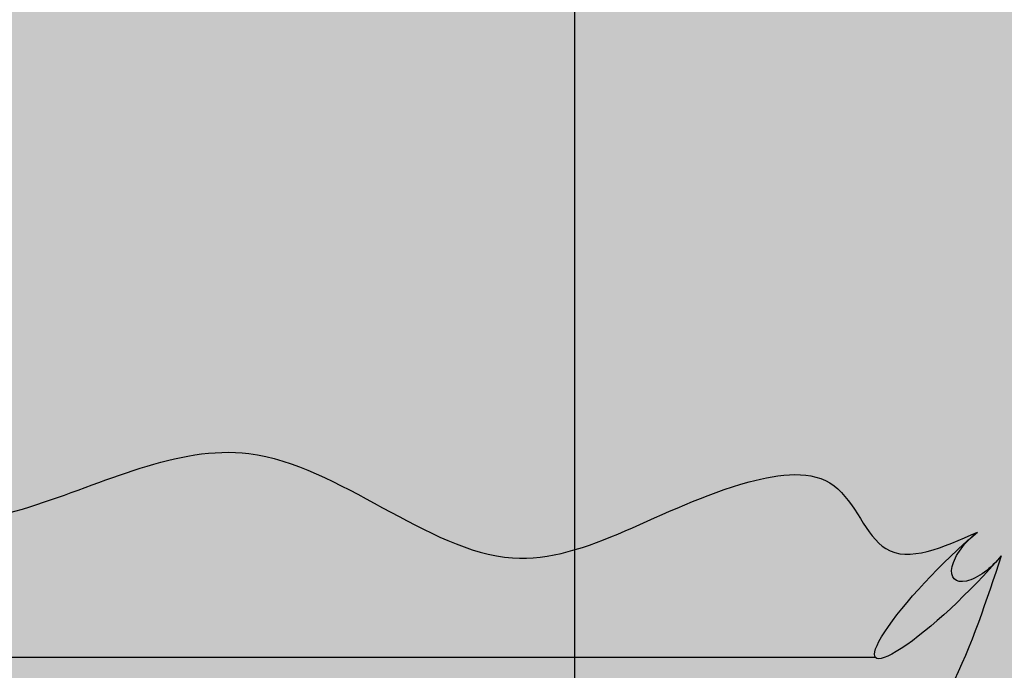
# Model space of a CAD drawing. Units: inches. Extents: x 1704 to 6393, y -157 to 1172.
# Tile 36 of 122: x 2526 to 2564, y 190 to 215. Entities that reach past the tile are written whole.
import ezdxf

# ---------------------------------------------------------------- set-up
doc = ezdxf.new("R2010")
doc.units = ezdxf.units.IN
doc.header["$MEASUREMENT"] = 0
for name, color, linetype, lineweight in [('A-ANNO-DIMS', 7, 'Continuous', 13), ('A-FURN', 8, 'Continuous', 18), ('estofado', 7, 'Continuous', 25)]:
    doc.layers.add(name, color=color, linetype=linetype, lineweight=lineweight)
doc.layers.add('A-FLOR-PATT', color=7, linetype='Continuous', lineweight=13, true_color=0xf2f2f2)
doc.styles.get("Standard").update_dxf_attribs({"font": 'arial.ttf'})
doc.dimstyles.get("Standard").update_dxf_attribs({"dimtxt": 6, "dimasz": 2, "dimexe": 0.18, "dimexo": 0.0625, "dimgap": 0.09, "dimtad": 0, "dimtih": 1, "dimtoh": 1, "dimdec": 1, "dimzin": 0, "dimdsep": 46, "dimlunit": 3, "dimtxsty": 'Standard', "dimblk": 'ARCHTICK', "dimcen": 0.09, "dimadec": 0, "dimazin": 0, "dimtfac": 1, "dimtdec": 1, "dimtofl": 0, "dimtmove": 0, "dimatfit": 3, "dimfxl": 1, "dimtolj": 1, "dimtzin": 0, "dimarcsym": 0})

# ---------------------------------------------------------------- blocks, each defined once
blk = doc.blocks.new('Cama Box Regencia LOLA')
at = {"layer": 'estofado', "ltscale": 0.2}
h = blk.add_hatch(color=256, dxfattribs=at)
h.dxf.hatch_style = 1
h.set_gradient(color1=(206, 178, 131), color2=(233, 221, 200), one_color=1, tint=0.8500000238418579, name='CURVED')
edge = h.paths.add_edge_path()
edge.add_spline(control_points=[(0.9233883396182136, -2.254908822900802), (0.9143712174658276, -2.237158585978875), (0.8971704820246486, -2.20329887728792), (0.9295105801843419, -2.140290914518345), (0.848651568119294, -2.10957861148239), (0.9047062348403186, -2.046222426005954), (0.8299480774321636, -1.990932361540615), (0.9387479200587449, -1.92692496801726), (0.8590435458045249, -1.86767849203585), (0.8322262745575699, -1.826028043643361), (0.8247981799574972, -1.810442049687992)], knot_values=[0, 0, 0, 0, 0.0575832900035364, 0.1098437972159638, 0.1698138218664432, 0.2255174829302509, 0.2824861515521905, 0.3632291183773252, 0.4509842065695901, 0.5012091817853866, 0.5012091817853866, 0.5012091817853866, 0.5012091817853866], degree=3, periodic=0)
edge.add_spline(control_points=[(0.8247981799572698, -1.810442049688447), (0.8512430237993839, -1.769990096378137), (0.8869160776755506, -1.705010622333873), (0.9070359522544322, -1.586338752195842), (0.8536462472426364, -1.488247672851343), (0.8944567470317679, -1.387739666353695), (0.8643796102055603, -1.342420998864781), (0.8547271521993025, -1.327877176513538)], knot_values=[0, 0, 0, 0, 0.1438744691785906, 0.2224893870322766, 0.3492927143212738, 0.4561786976395368, 0.5066917301592304, 0.5066917301592304, 0.5066917301592304, 0.5066917301592304], degree=3, periodic=0)
edge.add_spline(control_points=[(0.8547271521993025, -1.327877176513538), (0.7873766543807506, -1.256744909425322), (0.6449024721503065, -1.106270719748692), (0.3977250465933366, -1.412092721352792), (0.0338148848931041, -1.279726484458706), (-0.3488365122128698, -1.179158668568902), (-0.6188339616464873, -1.25080943574278), (-0.7460155200169539, -1.321708019985464)], knot_values=[0.0991852523588446, 0.0991852523588446, 0.0991852523588446, 0.0991852523588446, 0.3453008654366167, 0.6198216521345741, 0.9826525916749167, 1.386093159660275, 1.810554634340498, 1.810554634340498, 1.810554634340498, 1.810554634340498], degree=3, periodic=0)
edge.add_spline(control_points=[(-0.7460155199962628, -1.32170802000337), (-0.8056354908857201, -1.352141651537124), (-0.8226532004149476, -1.367823298399059), (-0.8348745804664758, -1.38184410903591)], knot_values=[0.0062456970656236, 0.0062456970656236, 0.0062456970656236, 0.0062456970656236, 0.0554759259147193, 0.0554759259147193, 0.0554759259147193, 0.0554759259147193], degree=3, periodic=0)
edge.add_spline(control_points=[(-0.8348745804664758, -1.38184410903591), (-0.8364250716851984, -1.383622888820184), (-0.8378983647115774, -1.385374937005849), (-0.8393716577378427, -1.387126985191514)], knot_values=[0, 0, 0, 0, 0.0062456970656236, 0.0062456970656236, 0.0062456970656236, 0.0062456970656236], degree=3, periodic=0)
edge.add_arc((-0.6180450437709624, -1.576392779500167), 0.2912164331649039, 139.4648411061637, 203.3711573294546)
edge.add_arc((-0.7011750866292914, -1.609837078845487), 0.2016528082906132, 204.0179006417974, 212.6189639884946)
edge.add_spline(control_points=[(-0.8710220093900034, -1.718537943240505), (-0.8696870122217887, -1.721658691442996), (-0.8597709916446092, -1.746046247230935), (-0.8464685798230674, -1.804421032451443), (-0.888988689927828, -1.889951451602371), (-0.8378676506146121, -1.973422824210047), (-0.8371590179440318, -2.05992368952792), (-0.8871569320951948, -2.144598622072578), (-0.908935644436724, -2.210906123939594), (-0.9233883398977695, -2.254908823284267)], knot_values=[0, 0, 0, 0, 0.0101500649009363, 0.0785829584511912, 0.1732273504791735, 0.2688802694005398, 0.3498050162211252, 0.4202002266429896, 0.5590752189863636, 0.5590752189863636, 0.5590752189863636, 0.5590752189863636], degree=3, periodic=0)
edge.add_ellipse((-0.9040800600764669, -2.258882422916315), major_axis=(0.0267880171833212, 0.0267880171833213), ratio=0.4535320972039226, start_angle=94.15910660291303, end_angle=123.37101895145429, ccw=False)
edge.add_ellipse((-0.8772920428931456, -2.232094405732993), major_axis=(0.0772920428927364, 0.0772920428927364), ratio=0.168252450050839, start_angle=-1.0527401173021644e-10, end_angle=156.3071135567154, ccw=False)
edge.add_line((-0.8000000000002955, -2.154802362840428), (0.7999592378284888, -2.154802362840428))
edge.add_arc((0.9462065466516378, -2.098298447668867), 0.1567831871334379, 200.9447658774159, 201.1244713640487, ccw=False)
edge.add_arc((1.115979327553759, -2.004946707326951), 0.3497136727815615, 205.2898146244752, 205.3730108333857)
edge.add_ellipse((0.8772920428930319, -2.232094405732993), major_axis=(-0.0772920428927364, 0.0772920428927364), ratio=0.168252450050839, start_angle=203.6928864432847, end_angle=359.99999999994674, ccw=False)
edge.add_ellipse((0.9040800600763532, -2.258882422916315), major_axis=(-0.0267880171833213, 0.0267880171833213), ratio=0.4535320972039226, start_angle=236.6289810485458, end_angle=265.84089339708703, ccw=False)
h = blk.add_hatch(color=256, dxfattribs=at)
h.dxf.hatch_style = 1
h.set_gradient(color1=(206, 178, 131), color2=(233, 221, 200), one_color=1, tint=0.8500000238418579, name='CURVED')
edge = h.paths.add_edge_path()
edge.add_ellipse((-0.8772920428931456, -2.232094405732993), major_axis=(0.0772920428927364, 0.0772920428927364), ratio=0.168252450050839, start_angle=-156.3071135577263, end_angle=-1.05349e-10)
edge.add_ellipse((-0.8772920428931456, -2.232094405732993), major_axis=(0.0772920428927364, 0.0772920428927364), ratio=0.168252450050839, start_angle=-1.05349e-10, end_angle=156.3071135567153)
edge.add_ellipse((-0.9040800600764669, -2.258882422916315), major_axis=(0.0267880171833212, 0.0267880171833213), ratio=0.4535320972039226, start_angle=-94.15910660848522, end_angle=94.15910660291303, ccw=False)
h = blk.add_hatch(color=256, dxfattribs=at)
h.dxf.hatch_style = 1
h.set_gradient(color1=(206, 178, 131), color2=(233, 221, 200), one_color=1, tint=0.8500000238418579, name='CURVED')
edge = h.paths.add_edge_path()
edge.add_spline(control_points=[(-0.9001064604443627, -2.27819070273756), (-0.866259371332262, -2.263084355976445), (-0.8028331991894219, -2.234776522858453), (-0.7685206103102474, -2.343981002846874), (-0.6122536186376238, -2.322828464485212), (-0.4353754265674752, -2.183795504726106), (-0.2043351766035357, -2.412166101990749), (0.035742157155596, -2.28434544697319), (0.2724023732024534, -2.265741378418681), (0.4990197572961961, -2.339647395113615), (0.6925408411253784, -2.202138696866825), (0.8240737498149427, -2.250332331133733), (0.900106460444249, -2.27819070273756)], knot_values=[0, 0, 0, 0, 0.0915194039844232, 0.1714985135733706, 0.2551966802733756, 0.4993431682155844, 0.7776132872898075, 0.9991109890269537, 1.23769004728933, 1.492615491211055, 1.658192352121012, 1.885025012049534, 1.885025012049534, 1.885025012049534, 1.885025012049534], degree=3, periodic=0)
edge.add_ellipse((0.9040800600763532, -2.258882422916315), major_axis=(-0.0267880171833213, 0.0267880171833213), ratio=0.4535320972039226, start_angle=454.1591066084853, end_angle=483.3710189511271, ccw=False)
edge.add_ellipse((0.8772920428930319, -2.232094405732993), major_axis=(-0.0772920428927364, 0.0772920428927364), ratio=0.168252450050839, start_angle=359.99999999994674, end_angle=516.3071135577263, ccw=False)
edge.add_arc((0.9462065466977946, -2.098298447788181), 0.1567831871334379, 201.1244713173118, 201.142614633458, ccw=False)
edge.add_line((0.7999592378286025, -2.154802362840428), (-0.8000000000004092, -2.154802362840428))
edge.add_ellipse((-0.8772920428931456, -2.232094405732993), major_axis=(0.0772920428927364, 0.0772920428927364), ratio=0.168252450050839, start_angle=-156.3071135577261, end_angle=-1.0527401173021644e-10, ccw=False)
edge.add_ellipse((-0.9040800600764669, -2.258882422916315), major_axis=(0.0267880171833212, 0.0267880171833213), ratio=0.4535320972039226, start_angle=-123.3710189511271, end_angle=-94.15910660848522, ccw=False)
blk.add_line((-0.7999999999999546, -2.154802362840428), (0.8000000000000682, -2.154802362840428), dxfattribs=at)
at = {"layer": 'estofado', "ltscale": 0.2, "extrusion": (0, 0, -1)}
for centre, major_axis, ratio, start_param, end_param in [((-0.8772920428931456, -2.232094405732993), (0.0772920428927364, 0.0772920428927364), 0.168252450050839, 4.250341947992563, 8.31602866635556), ((-0.9040800600764669, -2.258882422916315), (0.0267880171833212, 0.0267880171833213), 0.4535320972039226, 4.422106649467695, 8.144263964888069)]:
    blk.add_ellipse(centre, major_axis=major_axis, ratio=ratio, start_param=start_param, end_param=end_param, dxfattribs=at)
at = {"layer": 'estofado', "ltscale": 0.2}
for points, knots in [([(-0.9233883398977695, -2.254908823284267), (-0.908935644436724, -2.210906123939594), (-0.8871569320951948, -2.144598622072578), (-0.8371590179440318, -2.05992368952792), (-0.8378676506146121, -1.973422824210047), (-0.888988689927828, -1.889951451602371), (-0.8464685798230674, -1.804421032451443), (-0.8597709916446092, -1.746046247230935), (-0.8696870122217887, -1.721658691442996), (-0.8710220093900034, -1.718537943240505)], [0, 0, 0, 0, 0.1388749923433741, 0.2092702027652384, 0.2901949495858238, 0.3858478685071901, 0.4804922605351724, 0.5489251540854273, 0.5590752189863636, 0.5590752189863636, 0.5590752189863636, 0.5590752189863636]), ([(0.900106460444249, -2.27819070273756), (0.8240737498147286, -2.250332331133789), (0.6925408411252015, -2.202138696866918), (0.4990197572963532, -2.33964739511349), (0.2724023732023884, -2.265741378418779), (0.0357421571555867, -2.284345446973105), (-0.204335176603578, -2.412166101990773), (-0.4353754265674596, -2.183795504726199), (-0.6122536186375224, -2.322828464485116), (-0.7685206103102122, -2.343981002846907), (-0.8028331991894692, -2.234776522858419), (-0.8662593713322198, -2.263084355976456), (-0.9001064604443627, -2.27819070273756)], [0, 0, 0, 0, 0.2268326599285221, 0.3924095208384793, 0.6473349647602045, 0.8859140230225809, 1.107411724759727, 1.38568184383395, 1.629828331776159, 1.713526498476164, 1.793505608065111, 1.885025012049534, 1.885025012049534, 1.885025012049534, 1.885025012049534])]:
    blk.add_open_spline(points, degree=3, knots=knots, dxfattribs=at)
blk = doc.blocks.new('_ArchTick')
at = {"color": 0, "linetype": 'ByBlock', "const_width": 0.15}
blk.add_lwpolyline([(-0.5, -0.5), (0.5, 0.5)], dxfattribs=at)
blk = doc.blocks.new('*D93')
at = {"layer": 'A-ANNO-DIMS', "color": 0, "lineweight": -2, "transparency": 16777216}
for p, q in [((2605.286074000001, 895.2129740000005), (1829.697551000002, 895.2129740000003)), ((1829.877551000002, 895.2129740000003), (1829.877551000002, 495.8664119263302)), ((1829.877551000002, 90.2129739999999), (1829.877551000002, 489.5595360736699)), ((2605.286074000001, 90.21297400000003), (1829.697551000002, 90.2129739999999))]:
    blk.add_line(p, q, dxfattribs=at)
at = {"layer": 'Defpoints', "color": 0, "lineweight": -3, "transparency": 16777216}
for p in [(2605.348574000001, 895.2129740000005), (1829.877551000002, 90.2129739999999), (2605.348574000001, 90.21297400000003)]:
    blk.add_point(p, dxfattribs=at)
at = {"layer": 'A-ANNO-DIMS', "color": 0, "lineweight": -2, "transparency": 16777216, "xscale": 2, "yscale": 2, "zscale": 2}
for p, rotation in [((1829.877551000002, 895.2129740000003), 90), ((1829.877551000002, 90.2129739999999), 270)]:
    blk.add_blockref('_ArchTick', p, dxfattribs=dict(at, rotation=rotation))
at = {"layer": 'A-ANNO-DIMS', "color": 0, "transparency": 16777216, "insert": (1829.877551000001, 492.7129739999994), "char_height": 6, "attachment_point": 5}
blk.add_mtext('\\A1;805', dxfattribs=at)
blk = doc.blocks.new('*D105')
at = {"layer": 'A-ANNO-DIMS', "color": 0, "lineweight": -2, "transparency": 16777216}
for p, q in [((2451.737975, 615.150474), (2451.737975, -64.9670259999999)), ((2547.348574, 615.150474), (2547.348574, -64.9670259999999)), ((2451.737975, -64.787026), (2489.908936164393, -64.787026)), ((2547.348574, -64.787026), (2509.177612835607, -64.787026))]:
    blk.add_line(p, q, dxfattribs=at)
at = {"layer": 'Defpoints', "color": 0, "lineweight": -3, "transparency": 16777216}
for p in [(2451.737975, 615.212974), (2547.348574, 615.212974), (2547.348574, -64.787026)]:
    blk.add_point(p, dxfattribs=at)
at = {"layer": 'A-ANNO-DIMS', "color": 0, "lineweight": -2, "transparency": 16777216, "xscale": 2, "yscale": 2, "zscale": 2, "rotation": 180}
blk.add_blockref('_ArchTick', (2451.737975, -64.787026), dxfattribs=at)
at = {"layer": 'A-ANNO-DIMS', "color": 0, "lineweight": -2, "transparency": 16777216, "xscale": 2, "yscale": 2, "zscale": 2}
blk.add_blockref('_ArchTick', (2547.348574, -64.787026), dxfattribs=at)
at = {"layer": 'A-ANNO-DIMS', "color": 0, "transparency": 16777216, "insert": (2499.5432745, -64.787026), "char_height": 6, "attachment_point": 5}
blk.add_mtext('\\A1;95.61', dxfattribs=at)

msp = doc.modelspace()

# ---------------------------------------------------------------- hatches: boundary and pattern name
at = {"layer": 'A-FLOR-PATT', "transparency": 33554528}
h = msp.add_hatch(color=256, dxfattribs=at)
h.dxf.hatch_style = 1
h.paths.add_polyline_path([(2325.348574056059, 863.2129735309796), (2325.348574056059, 887.2129735309796), (2263.348574056059, 887.2129735309796), (2167.348574056059, 887.2129735309794), (2081.348574056061, 887.2129735309792), (2081.348574056061, 719.2129735309785), (2277.348574056059, 719.2129735309787), (2277.348574056059, 711.2129735309788), (2277.348574056059, 372.212973530979), (2349.348574056059, 372.212973530979), (2381.348574056059, 372.2129735309789), (2381.348574056059, 364.2129735309789), (2353.348574056059, 364.2129735309789), (2353.348574056059, 270.2129735309788), (2381.348574056059, 270.2129735309788), (2381.348574056059, 266.2129735309788), (2357.348574056059, 266.2129735309788), (2357.348574056059, 98.21297353097884), (2381.348574056059, 98.21297353097897), (2385.181056550604, 98.21297353097884), (2386.482186711948, 98.21297353097884), (2424.21496140017, 98.21297353097884), (2425.516091561514, 98.21297353097884), (2429.348574056059, 98.21297353097897), (2597.348574056059, 98.21297353097884), (2597.348574056059, 146.2129735309788), (2597.348574056059, 218.2129735309788), (2597.348574056059, 266.2129735309788), (2423.348574056059, 266.2129735309788), (2423.348574056059, 270.2129735309788), (2473.348574056059, 270.2129735309788), (2473.348574056059, 294.2129735309789), (2477.348574056059, 294.2129735309789), (2477.348574056059, 270.2129735309788), (2547.348574056059, 270.2129735309788), (2547.348574056059, 364.2129735309788), (2477.348574056059, 364.2129735309788), (2477.348574056059, 318.2129735309788), (2473.348574056059, 318.2129735309787), (2473.348574056059, 364.2129735309789), (2423.348574056059, 364.2129735309788), (2423.348574056059, 372.2129735309788), (2469.348574056059, 372.2129735309788), (2469.348574056059, 459.2129735309789), (2469.348574056059, 538.2129735309788), (2350.348574056059, 538.2129735309788), (2350.348574056059, 565.7129735309788), (2358.348574056059, 565.7129735309788), (2358.348574056059, 545.2129735309788), (2420.348574056059, 545.2129735309788), (2420.348574056059, 610.2129735309788), (2358.348574056059, 610.2129735309788), (2358.348574056059, 589.7129735309788), (2350.348574056059, 589.7129735309788), (2350.348574056059, 615.2129735309788), (2425.348574056059, 615.2129735309788), (2425.348574056059, 607.2129735309788), (2425.348574056059, 546.2129735309788), (2469.348574056059, 546.2129735309788), (2514.34857405606, 546.212973530979), (2514.34857405606, 607.2129735309788), (2449.348574056059, 607.2129735309788), (2449.348574056059, 615.2129735309788), (2451.737974987759, 615.2129735309788), (2451.737974987759, 659.2129735309788), (2427.737974987759, 659.2129735309788), (2427.737974987759, 665.2129735309788), (2367.737974987758, 665.2129735309788), (2367.737974987758, 667.2129735309788), (2367.737974987758, 711.2129735309788), (2325.348574056059, 711.2129735309788), (2325.348574056059, 719.2129735309785), (2325.348574056059, 755.2129735309787), (2325.348574056059, 763.2129735309788)])
h.paths.add_polyline_path([(2233.85817000392, 822.532660166629, -0.1872470486944155), (2233.85817000392, 809.1396667958562), (2231.697030374885, 808.8044951349628, 0.0848927708004382), (2233.130501812631, 814.4858417746204), (2230.423974436808, 814.4858417746204, -0.1042581087707907), (2228.553363812687, 808.3129425443484), (2217.750790159711, 807.1555239386723, -0.2222222222222219), (2217.750790159711, 824.5168030238124), (2228.553363812687, 823.3593844181363, -0.1042581087707933), (2230.423974436808, 817.1864851878643), (2233.130501812631, 817.1864851878643, 0.08489277080044), (2231.697030374885, 822.8678318275219)], flags=16)
h.paths.add_polyline_path([(2213.621360876743, 833.1974425663823), (2213.621360876743, 798.4748843961024), (2156.047684459484, 798.4748843961034), (2156.047684459485, 833.1974425663813)], flags=16)
h.paths.add_polyline_path([(2203.931929661768, 848.0987249710489), (2205.089348267444, 837.2961513180724, -0.2222222222222264), (2187.728069182304, 837.2961513180724), (2188.88548778798, 848.0987249710485, -0.104258108770792), (2195.058387018252, 849.9693355951691), (2195.058387018252, 852.6758629709927, 0.084892770800438), (2189.377040378595, 851.2423915332469), (2189.712212039488, 853.4035311622828, -0.1872470486944166), (2203.105205410261, 853.4035311622828), (2203.440377071154, 851.2423915332469, 0.084892770800438), (2197.759030431496, 852.6758629709927), (2197.759030431496, 849.9693355951691, -0.1042581087707896)], flags=16)
h.paths.add_polyline_path([(2181.940976153924, 837.2961513180726, -0.2222222222222323), (2164.579697068783, 837.2961513180724), (2165.73711567446, 848.0987249710487, -0.1042581087707905), (2171.910014904732, 849.9693355951691), (2171.910014904732, 852.6758629709927, 0.0848927708004445), (2166.228668265074, 851.2423915332469), (2166.563839925967, 853.403531162283, -0.1872470486944096), (2179.95683329674, 853.4035311622828), (2180.292004957633, 851.2423915332465, 0.0848927708004458), (2174.610658317976, 852.6758629709927), (2174.610658317976, 849.9693355951691, -0.104258108770801), (2180.783557548248, 848.0987249710482)], flags=16)
h.paths.add_polyline_path([(2205.089348267444, 794.376175644412), (2203.931929661768, 783.5736019914364, -0.1042581087707934), (2197.759030431496, 781.7029913673155), (2197.759030431496, 778.9964639914921, 0.084892770800439), (2203.440377071154, 780.4299354292382), (2203.105205410261, 778.2687958002022, -0.1872470486944172), (2189.712212039488, 778.2687958002018), (2189.377040378595, 780.4299354292377, 0.0848927708004369), (2195.058387018252, 778.9964639914919), (2195.058387018252, 781.7029913673153, -0.1042581087707904), (2188.88548778798, 783.5736019914358), (2187.728069182304, 794.3761756444126, -0.2222222222222231)], flags=16)
h.paths.add_polyline_path([(2181.940976153924, 794.376175644412), (2180.783557548248, 783.5736019914364, -0.1042581087708008), (2174.610658317976, 781.7029913673153), (2174.610658317976, 778.9964639914921, 0.0848927708004458), (2180.292004957633, 780.4299354292382), (2179.95683329674, 778.268795800202, -0.1872470486944096), (2166.563839925967, 778.2687958002018), (2166.228668265074, 780.4299354292378, 0.0848927708004446), (2171.910014904732, 778.9964639914919), (2171.910014904732, 781.7029913673153, -0.1042581087707904), (2165.73711567446, 783.5736019914358), (2164.579697068783, 794.3761756444123, -0.2222222222222294)], flags=16)
h.paths.add_polyline_path([(2151.918255176517, 807.1555239386723), (2141.115681523541, 808.3129425443484, -0.1042581087707911), (2139.24507089942, 814.4858417746204), (2136.538543523597, 814.4858417746204, 0.08489277080044), (2137.972014961343, 808.8044951349626), (2135.810875332307, 809.1396667958562, -0.1872470486944109), (2135.810875332307, 822.5326601666285), (2137.972014961343, 822.8678318275221, 0.0848927708004416), (2136.538543523597, 817.1864851878643), (2139.24507089942, 817.1864851878643, -0.104258108770793), (2141.115681523541, 823.3593844181363), (2151.918255176517, 824.5168030238124, -0.2222222222222205)], flags=16)
h.paths.add_polyline_path([(2357.868011454448, 363.4102250290031), (2358.813881560335, 363.4102250290031, 0.7537604849588476)], flags=16)
h.paths.add_polyline_path([(2372.241054283868, 363.1167008961685), (2372.248110816919, 363.1167008961685), (2372.248110816919, 363.3425764997267), (2371.30224071103, 363.3425764997267), (2371.30224071103, 363.1392706554335, -1.360391292333951)], flags=16)
h.paths.add_polyline_path([(2371.309297244092, 272.7157694655011), (2371.30224071103, 272.7157694655011), (2371.30224071103, 272.4898938619428), (2372.248110816919, 272.4898938619428), (2372.248110816919, 272.6931997062759, -1.360391292393621)], flags=16)
h.paths.add_polyline_path([(2357.875067987504, 272.7157694655011), (2357.868011454452, 272.7157694655011), (2357.868011454452, 272.4898938619428), (2358.813881560341, 272.4898938619428), (2358.813881560341, 272.6931997062361, -1.360391292333948)], flags=16)
h.paths.add_polyline_path([(2353.768696905258, 363.0736921025416), (2376.347425366111, 363.0736921025416), (2376.347425366111, 272.7587782591281), (2353.768696905258, 272.7587782591281)], flags=16)
h.paths.add_polyline_path([(2354.772195947961, 362.0701930598379), (2375.343926323407, 362.0701930598379), (2375.343926323407, 273.7622773018316), (2354.772195947961, 273.7622773018318)], flags=0)
h.paths.add_polyline_path([(2357.868011454452, 363.3425764997267), (2358.813881560341, 363.3425764997266), (2358.813881560341, 363.1167008961684), (2357.868011454452, 363.1167008961684)], flags=16)
h.paths.add_polyline_path([(2359.287941640134, 359.1843485433627), (2359.287941640134, 360.0631949744305), (2370.828180631237, 360.0631949744362), (2370.828180631237, 359.1843485433769), (2374.332057422314, 359.1843485433812), (2374.332057422312, 358.4635369582513), (2372.835178716611, 358.4635369582524), (2372.835178716611, 357.5410357047662), (2374.332057422314, 357.5410357047678), (2374.332057422312, 356.8202241196381), (2372.835178716611, 356.820224119639), (2372.835178716611, 355.897722866153), (2374.332057422314, 355.8977228661546), (2374.332057422312, 355.1769112810248), (2372.835178716611, 355.1769112810259), (2372.835178716611, 354.2544100275397), (2374.332057422334, 354.2544100275415), (2374.332057422331, 353.5335984424117), (2372.835178716631, 353.5335984424126), (2372.835178716631, 352.6110971889265), (2374.332057422334, 352.6110971889282), (2374.332057422331, 351.8902856037984), (2372.835178716631, 351.8902856037993), (2372.835178716631, 350.9677843503132), (2374.332057422334, 350.967784350315), (2374.332057422331, 350.2469727651852), (2372.835178716631, 350.2469727651861), (2372.835178716631, 349.3244715117), (2374.332057422334, 349.3244715117017), (2374.332057422331, 348.603659926572), (2372.835178716631, 348.6036599265729), (2372.835178716631, 347.6811586730868), (2374.332057422334, 347.6811586730886), (2374.332057422331, 346.9603470879587), (2372.835178716631, 346.9603470879598), (2372.835178716631, 346.0378458344735), (2374.332057422334, 346.0378458344753), (2374.332057422331, 345.3170342493456), (2372.835178716631, 345.3170342493465), (2372.835178716631, 344.3945329958605), (2374.332057422334, 344.3945329958621), (2374.332057422331, 343.6737214107324), (2372.835178716631, 343.6737214107334), (2372.835178716631, 342.751220157247), (2374.332057422334, 342.7512201572489), (2374.332057422331, 342.0304085721191), (2372.835178716631, 342.03040857212), (2372.835178716631, 341.1079073186338), (2374.332057422334, 341.1079073186356), (2374.332057422331, 340.3870957335057), (2372.835178716631, 340.3870957335066), (2372.835178716631, 339.4645944800207), (2374.332057422334, 339.4645944800223), (2374.332057422331, 338.7437828948924), (2372.835178716648, 338.7437828948933), (2372.835178716648, 337.8212816414076), (2374.332057422334, 337.8212816414093), (2374.332057422331, 337.1004700562794), (2372.835178716648, 337.1004700562803), (2372.835178716648, 336.1779688027942), (2374.332057422334, 336.1779688027961), (2374.332057422331, 335.4571572176662), (2372.835178716648, 335.4571572176673), (2372.835178716648, 334.5346559641809), (2374.332057422334, 334.5346559641828), (2374.332057422331, 333.8138443790529), (2372.835178716648, 333.8138443790539), (2372.835178716648, 332.8913431255679), (2374.332057422334, 332.8913431255696), (2374.332057422331, 332.1705315404397), (2372.835178716648, 332.1705315404406), (2372.835178716648, 331.2480302869545), (2374.332057422334, 331.2480302869563), (2374.332057422331, 330.5272187018265), (2372.835178716648, 330.5272187018273), (2372.835178716648, 329.6047174483413), (2374.332057422334, 329.6047174483431), (2374.332057422331, 328.8839058632133), (2372.835178716648, 328.8839058632143), (2372.835178716648, 327.9614046097282), (2374.332057422334, 327.9614046097298), (2374.332057422331, 327.2405930246), (2372.835178716648, 327.2405930246009), (2372.835178716648, 326.3180917711149), (2374.332057422334, 326.3180917711167), (2374.332057422331, 325.5972801859869), (2372.835178716648, 325.5972801859877), (2372.835178716648, 324.6747789325016), (2374.332057422334, 324.6747789325034), (2374.332057422331, 323.9539673473736), (2372.835178716648, 323.9539673473746), (2372.835178716648, 323.0314660938884), (2374.332057422334, 323.0314660938901), (2374.332057422331, 322.3106545087603), (2372.835178716648, 322.3106545087613), (2372.835178716648, 321.3881532552753), (2374.332057422334, 321.388153255277), (2374.332057422331, 320.6673416701471), (2372.835178716648, 320.6673416701481), (2372.835178716648, 319.7448404166621), (2374.332057422334, 319.7448404166638), (2374.332057422331, 319.0240288315339), (2372.835178716648, 319.0240288315348), (2372.835178716648, 318.1015275780487), (2374.332057422334, 318.1015275780504), (2374.332057422331, 317.3807159929205), (2372.835178716648, 317.3807159929214), (2372.835178716648, 316.4582147394357), (2374.332057422334, 316.4582147394373), (2374.332057422331, 315.7374031543073), (2372.835178716648, 315.7374031543084), (2372.835178716648, 314.8149019008223), (2374.332057422334, 314.8149019008241), (2374.332057422331, 314.0940903156943), (2372.835178716648, 314.0940903156952), (2372.835178716648, 313.171589062209), (2374.332057422334, 313.1715890622108), (2374.332057422331, 312.450777477081), (2372.835178716648, 312.4507774770819), (2372.835178716648, 311.5282762235959), (2374.332057422334, 311.5282762235977), (2374.332057422331, 310.8074646384678), (2372.835178716648, 310.8074646384687), (2372.835178716648, 309.8849633849827), (2374.332057422334, 309.8849633849844), (2374.332057422331, 309.1641517998546), (2372.835178716648, 309.1641517998555), (2372.835178716648, 308.2416505463693), (2374.332057422334, 308.2416505463712), (2374.332057422331, 307.5208389612412), (2372.835178716648, 307.5208389612421), (2372.835178716648, 306.5983377077562), (2374.332057422334, 306.598337707758), (2374.332057422331, 305.8775261226281), (2372.835178716648, 305.8775261226289), (2372.835178716648, 304.955024869143), (2374.332057422334, 304.9550248691447), (2374.332057422331, 304.2342132840149), (2372.835178716648, 304.2342132840158), (2372.835178716648, 303.3117120305298), (2374.332057422334, 303.3117120305316), (2374.332057422331, 302.5909004454018), (2372.835178716648, 302.5909004454027), (2372.835178716648, 301.6683991919165), (2374.332057422334, 301.6683991919183), (2374.332057422331, 300.9475876067885), (2372.835178716648, 300.9475876067894), (2372.835178716648, 300.0250863533033), (2374.332057422334, 300.025086353305), (2374.332057422331, 299.3042747681752), (2372.835178716648, 299.3042747681761), (2372.835178716648, 298.3817735146902), (2374.332057422334, 298.3817735146919), (2374.332057422331, 297.6609619295621), (2372.835178716648, 297.6609619295629), (2372.835178716648, 296.7384606760769), (2374.332057422334, 296.7384606760786), (2374.332057422331, 296.0176490909488), (2372.835178716648, 296.0176490909498), (2372.835178716648, 295.0951478374636), (2374.332057422334, 295.0951478374653), (2374.332057422331, 294.3743362523355), (2372.835178716648, 294.3743362523364), (2372.835178716648, 293.4518349988504), (2374.332057422334, 293.4518349988522), (2374.332057422331, 292.7310234137224), (2372.835178716648, 292.7310234137233), (2372.835178716648, 291.8085221602371), (2374.332057422334, 291.8085221602389), (2374.332057422331, 291.0877105751091), (2372.835178716648, 291.08771057511), (2372.835178716648, 290.165209321624), (2374.332057422334, 290.1652093216256), (2374.332057422331, 289.4443977364957), (2372.835178716648, 289.4443977364966), (2372.835178716648, 288.5218964830108), (2374.332057422334, 288.5218964830125), (2374.332057422331, 287.8010848978827), (2372.835178716648, 287.8010848978836), (2372.835178716648, 286.8785836443975), (2374.332057422334, 286.8785836443993), (2374.332057422331, 286.1577720592695), (2372.835178716648, 286.1577720592703), (2372.835178716648, 285.2352708057842), (2374.332057422334, 285.2352708057861), (2374.332057422331, 284.5144592206562), (2372.835178716648, 284.514459220657), (2372.835178716648, 283.5919579671712), (2374.332057422334, 283.5919579671728), (2374.332057422331, 282.871146382043), (2372.835178716648, 282.8711463820439), (2372.835178716648, 281.9486451285579), (2374.332057422334, 281.9486451285596), (2374.332057422331, 281.2278335434298), (2372.835178716648, 281.2278335434307), (2372.835178716648, 280.3053322899446), (2374.332057422334, 280.3053322899464), (2374.332057422331, 279.5845207048164), (2372.835178716648, 279.5845207048174), (2372.835178716648, 278.6620194513314), (2374.332057422334, 278.6620194513331), (2374.332057422331, 277.9412078662033), (2372.835178716648, 277.9412078662043), (2372.835178716648, 277.0187066127184), (2374.332057422334, 277.0187066127201), (2374.332057422331, 276.29789502759), (2370.828180631244, 276.2978950275922), (2370.828180631244, 275.7692753872335), (2359.287941640128, 275.7692753872392), (2359.287941640128, 276.2978950275993), (2355.784064849037, 276.2978950276015), (2355.784064849037, 277.0187066126971), (2357.280943554723, 277.0187066126989), (2357.280943554723, 277.9412078662137), (2355.784064849037, 277.9412078662145), (2355.784064849037, 278.6620194513103), (2357.280943554723, 278.6620194513122), (2357.280943554723, 279.5845207048271), (2355.784064849037, 279.584520704828), (2355.784064849037, 280.3053322899236), (2357.280943554723, 280.3053322899253), (2357.280943554723, 281.2278335434403), (2355.784064849037, 281.2278335434412), (2355.784064849037, 281.9486451285369), (2357.280943554723, 281.9486451285387), (2357.280943554723, 282.8711463820535), (2355.784064849037, 282.8711463820543), (2355.784064849037, 283.5919579671501), (2357.280943554723, 283.591957967152), (2357.280943554723, 284.5144592206668), (2355.784064849037, 284.5144592206676), (2355.784064849037, 285.2352708057632), (2357.280943554723, 285.2352708057651), (2357.280943554723, 286.1577720592801), (2355.784064849037, 286.1577720592809), (2355.784064849037, 286.8785836443766), (2357.280943554723, 286.8785836443784), (2357.280943554723, 287.8010848978931), (2355.784064849037, 287.8010848978941), (2355.784064849037, 288.5218964829895), (2357.280943554723, 288.5218964829913), (2357.280943554723, 289.4443977365064), (2355.784064849037, 289.4443977365072), (2355.784064849037, 290.1652093216029), (2357.280943554723, 290.1652093216047), (2357.280943554723, 291.0877105751197), (2355.784064849037, 291.0877105751206), (2355.784064849037, 291.8085221602161), (2357.280943554723, 291.8085221602179), (2357.280943554723, 292.7310234137328), (2355.784064849037, 292.7310234137337), (2355.784064849037, 293.4518349988293), (2357.280943554723, 293.451834998831), (2357.280943554723, 294.3743362523461), (2355.784064849037, 294.3743362523469), (2355.784064849037, 295.0951478374426), (2357.280943554723, 295.0951478374445), (2357.280943554723, 296.0176490909594), (2355.784064849037, 296.0176490909601), (2355.784064849037, 296.7384606760557), (2357.280943554723, 296.7384606760575), (2357.280943554723, 297.6609619295724), (2355.784064849037, 297.6609619295734), (2355.784064849037, 298.3817735146691), (2357.280943554723, 298.3817735146709), (2357.280943554723, 299.3042747681858), (2355.784064849037, 299.3042747681866), (2355.784064849037, 300.0250863532823), (2357.280943554723, 300.0250863532841), (2357.280943554723, 300.9475876067989), (2355.784064849037, 300.9475876067997), (2355.784064849037, 301.6683991918954), (2357.280943554723, 301.6683991918973), (2357.280943554723, 302.5909004454123), (2355.784064849037, 302.5909004454133), (2355.784064849037, 303.3117120305088), (2357.280943554723, 303.3117120305105), (2357.280943554723, 304.2342132840254), (2355.784064849037, 304.2342132840262), (2355.784064849037, 304.9550248691219), (2357.280943554723, 304.9550248691238), (2357.280943554723, 305.8775261226386), (2355.784064849037, 305.8775261226394), (2355.784064849037, 306.5983377077352), (2357.280943554723, 306.5983377077369), (2357.280943554723, 307.5208389612518), (2355.784064849037, 307.5208389612528), (2355.784064849037, 308.2416505463484), (2357.280943554723, 308.2416505463501), (2357.280943554723, 309.1641517998652), (2355.784064849037, 309.1641517998661), (2355.784064849037, 309.8849633849617), (2357.280943554723, 309.8849633849634), (2357.280943554723, 310.8074646384782), (2355.784064849037, 310.8074646384791), (2355.784064849037, 311.5282762235748), (2357.280943554723, 311.5282762235767), (2357.280943554723, 312.4507774770916), (2355.784064849037, 312.4507774770925), (2355.784064849037, 313.171589062188), (2357.280943554723, 313.1715890621898), (2357.280943554723, 314.0940903157049), (2355.784064849037, 314.0940903157058), (2355.784064849037, 314.8149019008013), (2357.280943554723, 314.8149019008032), (2357.280943554723, 315.7374031543179), (2355.784064849037, 315.7374031543187), (2355.784064849037, 316.4582147394146), (2357.280943554723, 316.4582147394165), (2357.280943554723, 317.3807159929311), (2355.784064849037, 317.3807159929321), (2355.784064849037, 318.1015275780277), (2357.280943554723, 318.1015275780295), (2357.280943554723, 319.0240288315445), (2355.784064849037, 319.0240288315454), (2355.784064849037, 319.744840416641), (2357.280943554723, 319.7448404166428), (2357.280943554723, 320.6673416701576), (2355.784064849037, 320.6673416701585), (2355.784064849037, 321.3881532552541), (2357.280943554723, 321.388153255256), (2357.280943554723, 322.3106545087708), (2355.784064849037, 322.3106545087718), (2355.784064849037, 323.0314660938674), (2357.280943554723, 323.0314660938692), (2357.280943554723, 323.9539673473843), (2355.784064849037, 323.9539673473851), (2355.784064849037, 324.6747789324806), (2357.280943554723, 324.6747789324824), (2357.280943554723, 325.5972801859974), (2355.784064849037, 325.5972801859983), (2355.784064849037, 326.3180917710939), (2357.280943554723, 326.3180917710958), (2357.280943554723, 327.2405930246105), (2355.784064849037, 327.2405930246113), (2355.784064849037, 327.9614046097071), (2357.280943554723, 327.961404609709), (2357.280943554723, 328.8839058632238), (2355.784064849037, 328.8839058632245), (2355.784064849037, 329.6047174483202), (2357.280943554723, 329.604717448322), (2357.280943554723, 330.527218701837), (2355.784064849037, 330.5272187018379), (2355.784064849037, 331.2480302869335), (2357.280943554723, 331.2480302869353), (2357.280943554723, 332.1705315404502), (2355.784064849037, 332.170531540451), (2355.784064849037, 332.8913431255468), (2357.280943554723, 332.8913431255486), (2357.280943554723, 333.8138443790634), (2355.784064849037, 333.8138443790642), (2355.784064849037, 334.5346559641599), (2357.280943554723, 334.5346559641618), (2357.280943554723, 335.4571572176767), (2355.784064849037, 335.4571572176776), (2355.784064849037, 336.1779688027732), (2357.280943554723, 336.177968802775), (2357.280943554723, 337.1004700562898), (2355.784064849037, 337.1004700562908), (2355.784064849037, 337.8212816413864), (2357.280943554723, 337.8212816413883), (2357.280943554723, 338.7437828949031), (2355.784064849037, 338.743782894904), (2355.784064849037, 339.4645944799996), (2357.280943554706, 339.4645944800013), (2357.280943554706, 340.3870957335163), (2355.784064849037, 340.3870957335173), (2355.784064849037, 341.1079073186129), (2357.280943554706, 341.1079073186146), (2357.280943554706, 342.0304085721296), (2355.784064849037, 342.0304085721304), (2355.784064849037, 342.7512201572262), (2357.280943554706, 342.751220157228), (2357.280943554706, 343.6737214107429), (2355.784064849037, 343.6737214107437), (2355.784064849037, 344.3945329958394), (2357.280943554706, 344.3945329958412), (2357.280943554706, 345.317034249356), (2355.784064849037, 345.3170342493569), (2355.784064849037, 346.0378458344526), (2357.280943554706, 346.0378458344544), (2357.280943554706, 346.9603470879692), (2355.784064849037, 346.9603470879701), (2355.784064849037, 347.6811586730658), (2357.280943554706, 347.6811586730677), (2357.280943554706, 348.6036599265824), (2355.784064849037, 348.6036599265833), (2355.784064849037, 349.324471511679), (2357.280943554706, 349.3244715116809), (2357.280943554706, 350.2469727651956), (2355.784064849037, 350.2469727651966), (2355.784064849037, 350.9677843502922), (2357.280943554706, 350.9677843502939), (2357.280943554706, 351.8902856038089), (2355.784064849037, 351.8902856038098), (2355.784064849037, 352.6110971889055), (2357.280943554706, 352.6110971889072), (2357.280943554706, 353.5335984424222), (2355.784064849037, 353.533598442423), (2355.784064849037, 354.2544100275187), (2357.280943554686, 354.2544100275204), (2357.280943554686, 355.1769112810354), (2355.784064849017, 355.1769112810362), (2355.784064849017, 355.897722866132), (2357.280943554686, 355.8977228661338), (2357.280943554686, 356.8202241196486), (2355.784064849017, 356.8202241196495), (2355.784064849017, 357.5410357047453), (2357.280943554686, 357.5410357047471), (2357.280943554686, 358.4635369582618), (2355.784064849017, 358.4635369582626), (2355.784064849017, 359.1843485433584)], flags=0)

# ---------------------------------------------------------------- block references
at = {"layer": 'A-FURN', "xscale": 39.22313671019584, "yscale": 39.22313671019584, "zscale": 39.22313671019584, "rotation": 180}
msp.add_blockref('Cama Box Regencia LOLA', (2527.569415053021, 106.0625493409584), dxfattribs=at)

# ---------------------------------------------------------------- dimensions: what is measured, and where the dimension line sits
at = {"layer": 'A-ANNO-DIMS'}
dim = msp.add_linear_dim(base=(1829.877551000002, 90.2129739999999), p1=(2605.348574000001, 895.212974), p2=(2605.348574000001, 90.21297399999999), angle=90, dimstyle='Standard', override={"dimdec": 0, "dimlfac": 1, "dimrnd": 0, "dimzin": 0, "dimdsep": 46, "dimlunit": 2}, dxfattribs=at)
dim.commit()
dim.dimension.update_dxf_attribs({"geometry": '*D93', "text_midpoint": (1829.877551000001, 492.7129739999994)})
dim = msp.add_linear_dim(base=(2547.348574, -64.787026), p1=(2451.737975, 615.212974), p2=(2547.348574, 615.212974), dimstyle='Standard', override={"dimdec": 2, "dimlfac": 1, "dimrnd": 0, "dimzin": 0, "dimdsep": 46, "dimlunit": 2}, dxfattribs=at)
dim.commit()
dim.dimension.update_dxf_attribs({"geometry": '*D105', "text_midpoint": (2499.5432745, -64.787026)})

doc.saveas('drawing.dxf')
